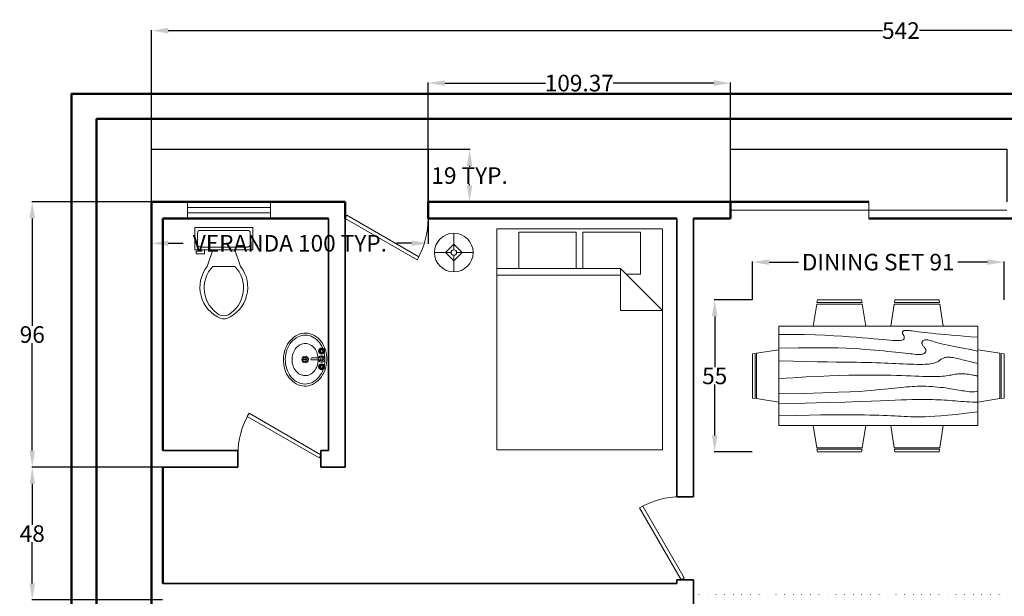
# Model space of a CAD drawing. Units: inches. Extents: x 910 to 1553, y 598 to 1516.
# Tile 5 of 6: x 912 to 1268, y 1307 to 1516. Entities that reach past the tile are written whole.
import ezdxf

# ---------------------------------------------------------------- set-up
doc = ezdxf.new("R2010")
doc.units = ezdxf.units.IN
doc.header["$MEASUREMENT"] = 0
doc.linetypes.add('ACAD_ISO07W100', pattern=[3, 0, -3])
for name, color, linetype, lineweight in [('A-ANNO-DIMS', 2, 'Continuous', 18), ('A-FLOR-BALC', 8, 'Continuous', 25), ('A-FLOR-OVHD', 8, 'ACAD_ISO07W100', 13), ('doors', 2, 'Continuous', 18), ('furniture', 11, 'Continuous', 18), ('Inner wall', 230, 'Continuous', 35), ('outer wall', 231, 'Continuous', 50), ('sanitory', 141, 'Continuous', 18), ('windows', 6, 'Continuous', 18)]:
    doc.layers.add(name, color=color, linetype=linetype, lineweight=lineweight)
doc.styles.get("Standard").update_dxf_attribs({"font": 'arial.ttf'})
doc.dimstyles.get("Standard").update_dxf_attribs({"dimtxt": 6, "dimasz": 6, "dimexe": 0.18, "dimexo": 0.0625, "dimgap": 0.09, "dimtad": 0, "dimtih": 1, "dimtoh": 1, "dimdec": 0, "dimzin": 0, "dimdsep": 46, "dimlunit": 3, "dimtxsty": 'Standard', "dimcen": 0.09, "dimadec": 0, "dimazin": 0, "dimtfac": 1, "dimtdec": 0, "dimtofl": 0, "dimtmove": 0, "dimatfit": 3, "dimfxl": 1, "dimtolj": 1, "dimtzin": 0, "dimarcsym": 0})

# ---------------------------------------------------------------- blocks, each defined once
blk = doc.blocks.new('*U5')
for p, q in [((0, 0), (0, -6)), ((-40, 0), (-40, -6))]:
    blk.add_line(p, q)
blk.add_lwpolyline([(0, 0), (-34.64, 20), (-35.52, 18.48), (-0.88, -1.52)], close=True)
blk.add_arc((0, 0), 40, 150, 180)
blk = doc.blocks.new('*U3')
for p, q in [((0, 0), (0, -6)), ((40, 0), (40, -6))]:
    blk.add_line(p, q)
blk.add_lwpolyline([(0, 0), (34.64, 20), (35.52, 18.48), (0.88, -1.52)], close=True)
blk.add_arc((0, 0), 40, 0, 30)
blk = doc.blocks.new('*U4')
for p, q in [((0, 0), (0, 6)), ((40, 0), (40, 6))]:
    blk.add_line(p, q)
blk.add_lwpolyline([(0, 0), (34.64, -20), (35.52, -18.48), (0.87, 1.52)], close=True)
blk.add_arc((0, 0), 40, 330, 0)
blk = doc.blocks.new('Faucet - Bathroom top')
for p, q in [((-4.107, 0.125), (-4.375, 0.125)), ((-3.75, 0.4788), (-3.75, 0.75)), ((-3.5, 0.482), (-3.5, 0.75)), ((-3.1461, 0.125), (-2.875, 0.125)), ((3.143, 0.125), (2.875, 0.125)), ((3.5, 0.4788), (3.5, 0.75)), ((3.75, 0.482), (3.75, 0.75)), ((4.1039, 0.125), (4.375, 0.125)), ((-4.1039, -0.125), (-4.375, -0.125)), ((-3.75, -0.4821), (-3.75, -0.75)), ((-3.5, -0.4789), (-3.5, -0.75)), ((-3.143, -0.125), (-2.875, -0.125)), ((-0.5, -0.8639), (-0.5, -4.5)), ((0.5, -4.5), (0.5, -0.8631)), ((3.1461, -0.125), (2.875, -0.125)), ((3.5, -0.4821), (3.5, -0.75)), ((3.75, -0.4789), (3.75, -0.75)), ((4.107, -0.125), (4.375, -0.125))]:
    blk.add_line(p, q)
for centre, radius in [((-3.625, 0), 1.375), ((-4.625, 0), 0.2795), ((-3.625, 0), 0.5), ((-3.625, 1), 0.2795), ((-2.625, 0), 0.2795), ((0, 0), 0.5), ((3.625, 0), 1.375), ((2.625, 0), 0.2795), ((3.625, 0), 0.5), ((3.625, 1), 0.2795), ((4.625, 0), 0.2795), ((-3.625, -1), 0.2795), ((3.625, -1), 0.2795)]:
    blk.add_circle(centre, radius)
for centre, radius, start, end in [((-3.625, 0), 1, 105.2407, 164.2093), ((-3.625, 0), 1, 16.44125, 74.07887), ((0, 0), 1.5, 289.6514, 250.3603), ((0, 0), 1, 300.3431, 239.7554), ((3.625, 0), 1, 106.12, 164.0884), ((3.625, 0), 1, 16.23422, 73.90469), ((-3.625, 0), 1, 196.2342, 253.9047), ((-3.625, 0), 1, 286.12, 344.0884), ((0, -4.5), 0.5, 180, 0), ((3.625, 0), 1, 196.4413, 254.0789), ((3.625, 0), 1, 285.2407, 344.2093)]:
    blk.add_arc(centre, radius, start, end)
blk = doc.blocks.new('Bed - Queen')
for p, q in [((0, -80.00003), (0, 0)), ((0, 0), (59.99999, 0)), ((59.99999, 0), (59.99999, -80.00003)), ((7.99999, -1.2), (28.79998, -1.2)), ((7.99999, -14.4), (7.99999, -1.2)), ((28.79998, -1.2), (28.79998, -14.4)), ((31.19999, -1.2), (51.99999, -1.2)), ((31.19999, -14.4), (31.19999, -1.2)), ((51.99999, -1.2), (51.99999, -16.4)), ((0, -14.4), (44.8, -14.4)), ((44.8, -16.8), (0, -16.8)), ((59.99999, -29.6), (44.8, -14.4)), ((44.8, -14.4), (44.8, -29.6)), ((51.99999, -16.4), (46.79936, -16.4)), ((44.8, -29.6), (59.99999, -29.6)), ((59.99999, -80.00003), (0, -80.00003))]:
    blk.add_line(p, q)
blk = doc.blocks.new('Lamp - Table')
for p, q in [((0, 7), (0, 1)), ((-1, 0), (-7, 0)), ((0, 3), (-3, 0)), ((-3, 0), (0, -3)), ((3, 0), (0, 3)), ((0, -3), (3, 0)), ((1, 0), (7, 0)), ((0, -1), (0, -7))]:
    blk.add_line(p, q)
for radius in [7, 1]:
    blk.add_circle((0, 0), radius)
blk = doc.blocks.new('Toilet - top')
for p, q in [((9.5, -6), (9.5, -2)), ((-10, -8.5), (-8, -8.5)), ((-10, -9.5), (-10, -8.5)), ((-7, -9.5), (-10, -9.5)), ((-8, -8.5), (-8, -8)), ((-7, -8), (-7, -9.5)), ((-4, -8), (-6, -14)), ((4, -8), (6, -14)), ((4, -14), (-4, -14))]:
    blk.add_line(p, q)
blk.add_lwpolyline([(10.5, -8), (10.5, 0), (-10.5, 0), (-10.5, -8)], close=True)
for points in [[(-9.5, -2), (-9.5, -6)], [(8.5, -1), (-8.5, -1)], [(-8.5, -7), (8.5, -7)]]:
    blk.add_lwpolyline(points)
for centre, radius, start, end in [((-8.62, -1.88), 0.884, 81.8699, 188.1301), ((8.62, -1.88), 0.884, 351.8699, 98.1301), ((-8.62, -6.12), 0.884, 171.8699, 278.1301), ((8.62, -6.12), 0.884, 261.8699, 8.1301), ((3.52, -21.58), 12.17, 141.4691, 247.9714), ((4.2, -21.82), 11.33, 136.3677, 238.9468), ((-3.52, -21.58), 12.17, 292.0284, 38.5307), ((-4.2, -21.82), 11.33, 301.053, 43.6321), ((0, -27.88), 4, 245.7318, 294.2682), ((0, -29), 4, 254.8605, 285.1395)]:
    blk.add_arc(centre, radius, start, end)
blk = doc.blocks.new('Dining Set - 36 x 72 in.')
for p, q in [((-22.2343, 26.00059), (-23.4847, 17.99762)), ((-22.2304, 26), (-5.7608, 26)), ((-22, 27.5), (-22.1562, 26.50042)), ((-5.8416, 26.5), (-22.1534, 26.5)), ((-22, 27.5), (-6, 27.5)), ((-5.8437, 26.49966), (-6, 27.5)), ((-4.5152, 17.99762), (-5.7655, 25.99926)), ((5.7657, 26.00059), (4.5153, 17.99762)), ((5.7696, 26), (22.2392, 26)), ((6, 27.5), (5.8438, 26.50042)), ((22.1584, 26.5), (5.8466, 26.5)), ((6, 27.5), (22, 27.5)), ((22.1563, 26.49966), (22, 27.5)), ((23.4848, 17.99762), (22.2345, 25.99926)), ((36, 18), (-36, 18)), ((-36, 18), (-36, -18)), ((36, -18), (36, 18)), ((-45.5, 8), (-44.5004, 8.15617)), ((-45.5, 8), (-45.5, -8)), ((-44.5, -8.15843), (-44.5, 8.15338)), ((-44.0006, 8.23428), (-35.9976, 9.48474)), ((-44, 8.23041), (-44, -8.23915)), ((44.0006, 8.23428), (35.9976, 9.48474)), ((44, 8.23041), (44, -8.23915)), ((44.5, -8.15843), (44.5, 8.15338)), ((45.5, 8), (44.5005, 8.15617)), ((45.5, 8), (45.5, -8)), ((-44.4997, -8.15631), (-45.5, -8)), ((-35.9976, -9.48476), (-43.9993, -8.2345)), ((35.9976, -9.48476), (43.9993, -8.2345)), ((44.4997, -8.15631), (45.5, -8)), ((-36, -18), (36, -18)), ((-22.2343, -26.0006), (-23.4847, -17.99762)), ((-4.5152, -17.99762), (-5.7655, -25.99928)), ((5.7657, -26.0006), (4.5153, -17.99762)), ((23.4848, -17.99762), (22.2345, -25.99928)), ((-22.2304, -26), (-5.7608, -26)), ((-22, -27.5), (-22.1562, -26.50044)), ((-5.8416, -26.5), (-22.1534, -26.5)), ((-22, -27.5), (-6, -27.5)), ((-5.8437, -26.49967), (-6, -27.5)), ((5.7696, -26), (22.2392, -26)), ((6, -27.5), (5.8438, -26.50044)), ((22.1584, -26.5), (5.8466, -26.5)), ((6, -27.5), (22, -27.5)), ((22.1563, -26.49967), (22, -27.5))]:
    blk.add_line(p, q)
for points in [[(-36, 15), (-31.1772, 14.97754), (-26.8079, 14.91406), (-22.8538, 14.81543), (-19.276, 14.6875), (-16.0362, 14.53613), (-13.0957, 14.36718), (-10.4159, 14.18652), (-7.9583, 14), (-5.6904, 13.81315), (-3.6035, 13.63021), (-1.6954, 13.45508), (0.0365, 13.29166), (1.5945, 13.14388), (2.9811, 13.01562), (4.1988, 12.9108), (5.25, 12.83333), (6.1393, 12.78613), (6.8802, 12.76823), (7.4883, 12.77767), (7.9792, 12.8125), (8.3685, 12.87077), (8.6719, 12.95052), (8.9049, 13.0498), (9.0833, 13.16666), (9.2205, 13.29899), (9.3216, 13.44401), (9.3895, 13.59879), (9.4271, 13.76041), (9.4373, 13.92594), (9.4232, 14.09245), (9.3875, 14.257), (9.3333, 14.41666), (9.2638, 14.56917), (9.1836, 14.71484), (9.0975, 14.85465), (9.0104, 14.98958), (8.9272, 15.1206), (8.8529, 15.2487), (8.7922, 15.37483), (8.75, 15.5), (8.7305, 15.62467), (8.7344, 15.74739), (8.7617, 15.86621), (8.8125, 15.97916), (8.8867, 16.08431), (8.9844, 16.17968), (9.1055, 16.26334), (9.25, 16.33333), (9.4189, 16.38802), (9.6172, 16.42708), (9.8506, 16.45052), (10.125, 16.45833), (10.4463, 16.45052), (10.8203, 16.42708), (11.2529, 16.38802), (11.75, 16.33333), (12.3184, 16.26318), (12.9694, 16.17838), (13.7151, 16.07991), (14.5677, 15.96875), (15.5395, 15.84586), (16.6426, 15.71224), (17.8893, 15.56884), (19.2917, 15.41666), (20.859, 15.25667), (22.5879, 15.08984), (24.4721, 14.91715), (26.5052, 14.73958), (28.6809, 14.5581), (30.9929, 14.3737), (33.4347, 14.18733), (36, 14)], [(-36, 10), (-28.9766, 10.14274), (-23.1725, 10.20442), (-18.4241, 10.19775), (-14.5677, 10.13541), (-11.4399, 10.03011), (-8.877, 9.89453), (-6.7154, 9.74137), (-4.7917, 9.58333), (-2.9698, 9.43082), (-1.2246, 9.28515), (0.4415, 9.14534), (2.026, 9.01041), (3.5266, 8.87939), (4.9408, 8.7513), (6.266, 8.62516), (7.5, 8.5), (8.6411, 8.37549), (9.6914, 8.2539), (10.6538, 8.13818), (11.5312, 8.03125), (12.3267, 7.93603), (13.043, 7.85547), (13.6831, 7.79248), (14.25, 7.75), (14.7471, 7.7303), (15.1797, 7.73307), (15.5537, 7.75732), (15.875, 7.80208), (16.1494, 7.86637), (16.3828, 7.94922), (16.5811, 8.04964), (16.75, 8.16666), (16.8944, 8.29915), (17.0143, 8.44531), (17.1089, 8.60319), (17.1771, 8.77083), (17.218, 8.94629), (17.2305, 9.1276), (17.2137, 9.31282), (17.1667, 9.5), (17.0895, 9.6875), (16.987, 9.875), (16.8649, 10.0625), (16.7292, 10.25), (16.5856, 10.4375), (16.4401, 10.625), (16.2985, 10.8125), (16.1667, 11), (16.05, 11.18733), (15.9518, 11.3737), (15.8752, 11.5581), (15.8229, 11.73958), (15.798, 11.91715), (15.8034, 12.08984), (15.842, 12.25667), (15.9167, 12.41666), (16.0295, 12.56836), (16.1784, 12.70833), (16.3605, 12.83268), (16.5729, 12.9375), (16.8127, 13.01888), (17.0768, 13.07291), (17.3625, 13.0957), (17.6667, 13.08333), (17.9894, 13.03312), (18.3418, 12.94726), (18.7382, 12.82918), (19.1927, 12.68229), (19.7195, 12.51001), (20.3327, 12.31575), (21.0465, 12.10294), (21.875, 11.875), (22.8357, 11.63354), (23.959, 11.37304), (25.2786, 11.08618), (26.8282, 10.76562), (28.6414, 10.40405), (30.752, 9.99414), (33.1936, 9.52856), (36, 9)], [(-36, 5.5), (-30.7157, 5.3348), (-26.069, 5.20963), (-21.9946, 5.11767), (-18.4271, 5.05208), (-15.3009, 5.00602), (-12.5508, 4.97265), (-10.1112, 4.94515), (-7.9167, 4.91666), (-5.909, 4.88167), (-4.0586, 4.83984), (-2.3429, 4.79215), (-0.7396, 4.73958), (0.7739, 4.6831), (2.22, 4.6237), (3.6213, 4.56233), (5, 4.5), (6.373, 4.43782), (7.7344, 4.3776), (9.0723, 4.32129), (10.375, 4.27083), (11.6309, 4.22819), (12.8281, 4.19531), (13.9551, 4.17415), (15, 4.16666), (15.954, 4.17448), (16.819, 4.19791), (17.6001, 4.23698), (18.3021, 4.29166), (18.9299, 4.36198), (19.4883, 4.44791), (19.9823, 4.54948), (20.4167, 4.66666), (20.7969, 4.79899), (21.1302, 4.94401), (21.4245, 5.09879), (21.6875, 5.26041), (21.9271, 5.42594), (22.1511, 5.59245), (22.3672, 5.757), (22.5834, 5.91666), (22.8065, 6.06868), (23.0404, 6.21093), (23.2879, 6.34147), (23.5521, 6.45833), (23.8358, 6.55957), (24.142, 6.64323), (24.4735, 6.70735), (24.8334, 6.75), (25.2235, 6.76969), (25.642, 6.76692), (26.0858, 6.74267), (26.5521, 6.69791), (27.0379, 6.63362), (27.5404, 6.55078), (28.0565, 6.45036), (28.5834, 6.33333), (29.1242, 6.19987), (29.7071, 6.04687), (30.3661, 5.87044), (31.1354, 5.66666), (32.0493, 5.43164), (33.142, 5.16146), (34.4475, 4.85221), (36, 4.5)], [(-36, -1), (-30.7915, -0.6591), (-26.0195, -0.38216), (-21.6519, -0.16284), (-17.6563, 0.00521), (-14.0005, 0.12833), (-10.6523, 0.21289), (-7.5796, 0.26522), (-4.75, 0.29166), (-2.134, 0.29793), (0.2878, 0.28711), (2.5317, 0.26163), (4.6146, 0.22396), (6.5529, 0.17651), (8.3633, 0.12174), (10.0623, 0.06209), (11.6667, 0), (13.1899, -0.06201), (14.6341, -0.1211), (15.9982, -0.17432), (17.2813, -0.21875), (18.4823, -0.25147), (19.6003, -0.26953), (20.6343, -0.27002), (21.5834, -0.25), (22.4481, -0.20768), (23.2357, -0.14584), (23.9549, -0.06836), (24.6146, 0.02083), (25.2235, 0.11784), (25.7904, 0.21875), (26.3241, 0.31966), (26.8334, 0.41666), (27.3265, 0.50618), (27.8099, 0.58593), (28.2894, 0.65397), (28.7709, 0.70833), (29.2601, 0.74707), (29.763, 0.76823), (30.2855, 0.76985), (30.8334, 0.75), (31.4088, 0.70784), (31.9994, 0.64713), (32.589, 0.57275), (33.1615, 0.48958), (33.7008, 0.4025), (34.1908, 0.3164), (34.6153, 0.23616), (34.9584, 0.16666), (35.2099, 0.11165), (35.3848, 0.07031), (35.504, 0.04069), (35.5886, 0.02083), (35.6594, 0.00879), (35.7377, 0.0026), (35.8442, 0.00032), (36, 0)], [(-36, -6.5), (-27.1843, -6.31267), (-20.084, -6.1263), (-14.469, -5.9419), (-10.1094, -5.76042), (-6.7752, -5.58285), (-4.2363, -5.41016), (-2.2629, -5.24333), (-0.625, -5.08334), (0.8708, -4.93099), (2.2715, -4.78646), (3.5872, -4.64974), (4.8281, -4.52084), (6.0046, -4.39974), (7.127, -4.28646), (8.2053, -4.18099), (9.25, -4.08334), (10.2705, -3.99382), (11.2734, -3.91407), (12.2647, -3.84603), (13.25, -3.79167), (14.2354, -3.75293), (15.2266, -3.73177), (16.2295, -3.73015), (17.25, -3.75), (18.2912, -3.79248), (19.3451, -3.85547), (20.4009, -3.93604), (21.4479, -4.03125), (22.4754, -4.13819), (23.4727, -4.25391), (24.4289, -4.37549), (25.3334, -4.5), (26.1785, -4.62492), (26.9694, -4.74935), (27.7145, -4.87281), (28.4219, -4.99479), (29.1, -5.11483), (29.7572, -5.23242), (30.4016, -5.34709), (31.0417, -5.45834), (31.6837, -5.56437), (32.3262, -5.65821), (32.9658, -5.73153), (33.599, -5.77604), (34.2224, -5.78345), (34.8327, -5.74545), (35.4264, -5.65373), (36, -5.5)], [(-36, -10), (-26.4022, -9.81299), (-18.4675, -9.62891), (-11.9839, -9.45069), (-6.7396, -9.28125), (-2.5226, -9.12354), (0.8789, -8.98047), (3.6769, -8.85498), (6.0833, -8.75), (8.2767, -8.66765), (10.3021, -8.60677), (12.1712, -8.56543), (13.8958, -8.54167), (15.4876, -8.53353), (16.9583, -8.53907), (18.3197, -8.55632), (19.5834, -8.58334), (20.7616, -8.61841), (21.8685, -8.66081), (22.9188, -8.71004), (23.9271, -8.76563), (24.9081, -8.82707), (25.8763, -8.89388), (26.8465, -8.96558), (27.8334, -9.04167), (28.8474, -9.12118), (29.8828, -9.20117), (30.93, -9.27824), (31.9792, -9.34896), (33.0205, -9.40991), (34.0443, -9.45768), (35.0407, -9.48885), (36, -9.5)], [(-36, -14.5), (-30.0881, -14.33513), (-25.0332, -14.21224), (-20.7312, -14.12647), (-17.0781, -14.07292), (-13.97, -14.04671), (-11.3027, -14.04297), (-8.9724, -14.05681), (-6.875, -14.08334), (-4.9224, -14.11833), (-3.0905, -14.16016), (-1.3709, -14.20785), (0.2448, -14.26042), (1.7647, -14.3169), (3.1973, -14.3763), (4.5507, -14.43767), (5.8333, -14.5), (7.0554, -14.5621), (8.235, -14.62175), (9.3922, -14.67652), (10.5469, -14.72396), (11.7192, -14.76164), (12.929, -14.78711), (14.1965, -14.79794), (15.5417, -14.79167), (16.9933, -14.76424), (18.6152, -14.70508), (20.4804, -14.60197), (22.6615, -14.44271), (25.2312, -14.21509), (28.2624, -13.9069), (31.8277, -13.50594), (36, -13)]]:
    blk.add_lwpolyline(points)
blk = doc.blocks.new('Sink - Oval top')
for p, q in [((-1, 0), (1, 0)), ((0, 1), (0, -1))]:
    blk.add_line(p, q)
for points in [[(-12.23, 0.39, 0.117634), (-11.46, -3.36, 0.104469), (-8.88, -6.8, 0.090016), (-5.08, -9.07, 0.08192), (-0.32, -10.02, 0.08192), (4.49, -9.38, 0.090016), (8.42, -7.36, 0.104469), (11.22, -4.09, 0.117634), (12.23, -0.39, 0.117634), (11.46, 3.36, 0.104469), (8.88, 6.8, 0.090016), (5.08, 9.07, 0.08192), (0.32, 10.02, 0.08192), (-4.49, 9.38, 0.090016), (-8.42, 7.36, 0.104469), (-11.22, 4.09, 0.117634)], [(-11.29, 0.16, 0.118622), (-10.52, -3.25, 0.104678), (-8.07, -6.36, 0.089562), (-4.54, -8.37, 0.081185), (-0.13, -9.15, 0.081185), (4.3, -8.49, 0.089562), (7.89, -6.58, 0.104678), (10.42, -3.55, 0.118622), (11.29, -0.16, 0.118622), (10.52, 3.25, 0.104678), (8.07, 6.36, 0.089562), (4.54, 8.37, 0.081185), (0.13, 9.15, 0.081185), (-4.3, 8.49, 0.089562), (-7.89, 6.58, 0.104678), (-10.42, 3.55, 0.118622)], [(-7.42, 0.08, 0.118283), (-6.91, -2.17, 0.104607), (-5.29, -4.21, 0.089718), (-2.97, -5.53, 0.081436), (-0.07, -6.04, 0.081436), (2.84, -5.59, 0.089718), (5.2, -4.33, 0.104607), (6.86, -2.32, 0.118283), (7.42, -0.08, 0.118283), (6.91, 2.17, 0.104607), (5.29, 4.21, 0.089718), (2.97, 5.53, 0.081436), (0.07, 6.04, 0.081436), (-2.84, 5.59, 0.089718), (-5.2, 4.33, 0.104607), (-6.86, 2.32, 0.118283)]]:
    blk.add_lwpolyline(points, format="xyb", close=True)
for radius in [1.5, 1]:
    blk.add_circle((0, 0), radius)
blk = doc.blocks.new('WIN-30X6')
for p, q in [((0, 6), (30, 6)), ((0, 0), (0, 6)), ((0, 4), (30, 4)), ((30, 6), (30, 0)), ((30, 2), (0, 2)), ((30, 0), (0, 0))]:
    blk.add_line(p, q)
blk = doc.blocks.new('VERANDA-EDGE-SHALLOW')
for p, q in [((0, 0), (0, 18.99)), ((0, 18.99), (100, 18.99)), ((100, 18.99), (100, 0))]:
    blk.add_line(p, q)
blk = doc.blocks.new('*D45')
at = {"layer": 'A-ANNO-DIMS', "color": 0, "lineweight": -2, "transparency": 16777216}
for p, q in [((959.7, 1449.91), (959.7, 1434.79)), ((1059.7, 1449.91), (1059.7, 1434.79)), ((965.7, 1434.97), (971.1, 1434.97)), ((1053.7, 1434.97), (1048.31, 1434.97))]:
    blk.add_line(p, q, dxfattribs=at)
for points in [[(965.7, 1435.97), (965.7, 1433.97), (959.7, 1434.97)], [(1053.7, 1435.97), (1053.7, 1433.97), (1059.7, 1434.97)]]:
    blk.add_solid(points, dxfattribs=at)
at = {"layer": 'Defpoints', "color": 0, "lineweight": -2, "transparency": 16777216}
for p in [(959.7, 1449.97), (1059.7, 1449.97), (1059.7, 1434.97)]:
    blk.add_point(p, dxfattribs=at)
at = {"layer": 'A-ANNO-DIMS', "color": 0, "transparency": 16777216, "insert": (1009.7, 1434.97), "char_height": 6, "attachment_point": 5}
blk.add_mtext('\\A1;VERANDA 100 TYP.', dxfattribs=at)
blk = doc.blocks.new('*D46')
at = {"layer": 'A-ANNO-DIMS', "color": 0, "lineweight": -2, "transparency": 16777216}
for p, q in [((1059.76, 1468.95), (1074.88, 1468.95)), ((1074.7, 1462.95), (1074.7, 1462.62)), ((1074.7, 1455.97), (1074.7, 1456.31)), ((1059.76, 1449.97), (1074.88, 1449.97))]:
    blk.add_line(p, q, dxfattribs=at)
for points in [[(1073.7, 1462.95), (1075.7, 1462.95), (1074.7, 1468.95)], [(1073.7, 1455.97), (1075.7, 1455.97), (1074.7, 1449.97)]]:
    blk.add_solid(points, dxfattribs=at)
at = {"layer": 'Defpoints', "color": 0, "lineweight": -2, "transparency": 16777216}
for p in [(1059.7, 1468.95), (1074.7, 1468.95), (1059.7, 1449.97)]:
    blk.add_point(p, dxfattribs=at)
at = {"layer": 'A-ANNO-DIMS', "color": 0, "transparency": 16777216, "insert": (1074.7, 1459.46), "char_height": 6, "attachment_point": 5}
blk.add_mtext('\\A1;19 TYP.', dxfattribs=at)
blk = doc.blocks.new('*D53')
at = {"layer": 'A-ANNO-DIMS', "color": 0, "lineweight": -2, "transparency": 16777216}
for p, q in [((1177, 1414.56), (1177, 1428.33)), ((1183, 1428.15), (1193.69, 1428.15)), ((1262, 1428.15), (1251.31, 1428.15)), ((1268, 1414.56), (1268, 1428.33))]:
    blk.add_line(p, q, dxfattribs=at)
for points in [[(1183, 1429.15), (1183, 1427.15), (1177, 1428.15)], [(1262, 1429.15), (1262, 1427.15), (1268, 1428.15)]]:
    blk.add_solid(points, dxfattribs=at)
at = {"layer": 'Defpoints', "color": 0, "lineweight": -2, "transparency": 16777216}
for p in [(1268, 1428.15), (1177, 1414.5), (1268, 1414.5)]:
    blk.add_point(p, dxfattribs=at)
at = {"layer": 'A-ANNO-DIMS', "color": 0, "transparency": 16777216, "insert": (1222.5, 1428.15), "char_height": 6, "attachment_point": 5}
blk.add_mtext('\\A1;DINING SET 91', dxfattribs=at)
blk = doc.blocks.new('*D54')
at = {"layer": 'A-ANNO-DIMS', "color": 0, "lineweight": -2, "transparency": 16777216}
for p, q in [((1176.94, 1414.5), (1163.17, 1414.5)), ((1163.35, 1408.5), (1163.35, 1390.14)), ((1163.35, 1365.5), (1163.35, 1383.86)), ((1176.94, 1359.5), (1163.17, 1359.5))]:
    blk.add_line(p, q, dxfattribs=at)
for points in [[(1162.35, 1408.5), (1164.35, 1408.5), (1163.35, 1414.5)], [(1162.35, 1365.5), (1164.35, 1365.5), (1163.35, 1359.5)]]:
    blk.add_solid(points, dxfattribs=at)
at = {"layer": 'Defpoints', "color": 0, "lineweight": -2, "transparency": 16777216}
for p in [(1163.35, 1414.5), (1177, 1414.5), (1177, 1359.5)]:
    blk.add_point(p, dxfattribs=at)
at = {"layer": 'A-ANNO-DIMS', "color": 0, "transparency": 16777216, "insert": (1163.35, 1387), "char_height": 6, "attachment_point": 5}
blk.add_mtext('\\A1;55', dxfattribs=at)
blk = doc.blocks.new('*D55')
at = {"layer": 'A-ANNO-DIMS', "color": 0, "lineweight": -2, "transparency": 16777216}
for p, q in [((959.7, 1469.02), (959.7, 1512.08)), ((965.7, 1511.9), (1224.01, 1511.9)), ((1495.7, 1511.9), (1237.39, 1511.9)), ((1501.7, 1469.02), (1501.7, 1512.08))]:
    blk.add_line(p, q, dxfattribs=at)
for points in [[(965.7, 1512.9), (965.7, 1510.9), (959.7, 1511.9)], [(1495.7, 1512.9), (1495.7, 1510.9), (1501.7, 1511.9)]]:
    blk.add_solid(points, dxfattribs=at)
at = {"layer": 'Defpoints', "color": 0, "lineweight": -2, "transparency": 16777216}
for p in [(1501.7, 1511.9), (959.7, 1468.95), (1501.7, 1468.95)]:
    blk.add_point(p, dxfattribs=at)
at = {"layer": 'A-ANNO-DIMS', "color": 0, "transparency": 16777216, "insert": (1230.7, 1511.9), "char_height": 6, "attachment_point": 5}
blk.add_mtext('\\A1;542', dxfattribs=at)
blk = doc.blocks.new('*D69')
at = {"layer": 'A-ANNO-DIMS', "color": 0, "lineweight": -2, "transparency": 16777216}
for p, q in [((963.64, 1353.97), (916.34, 1353.97)), ((916.52, 1347.97), (916.52, 1333.12)), ((916.52, 1311.97), (916.52, 1326.82)), ((963.64, 1305.97), (916.34, 1305.97))]:
    blk.add_line(p, q, dxfattribs=at)
for points in [[(915.52, 1347.97), (917.52, 1347.97), (916.52, 1353.97)], [(915.52, 1311.97), (917.52, 1311.97), (916.52, 1305.97)]]:
    blk.add_solid(points, dxfattribs=at)
at = {"layer": 'Defpoints', "color": 0, "lineweight": -2, "transparency": 16777216}
for p in [(916.52, 1353.97), (963.7, 1353.97), (963.7, 1305.97)]:
    blk.add_point(p, dxfattribs=at)
at = {"layer": 'A-ANNO-DIMS', "color": 0, "transparency": 16777216, "insert": (916.52, 1329.97), "char_height": 6, "attachment_point": 5}
blk.add_mtext('\\A1;48', dxfattribs=at)
blk = doc.blocks.new('*D70')
at = {"layer": 'A-ANNO-DIMS', "color": 0, "lineweight": -2, "transparency": 16777216}
for p, q in [((959.64, 1449.97), (916.34, 1449.97)), ((916.52, 1443.97), (916.52, 1405.12)), ((916.52, 1359.97), (916.52, 1398.82)), ((963.64, 1353.97), (916.34, 1353.97))]:
    blk.add_line(p, q, dxfattribs=at)
for points in [[(915.52, 1443.97), (917.52, 1443.97), (916.52, 1449.97)], [(915.52, 1359.97), (917.52, 1359.97), (916.52, 1353.97)]]:
    blk.add_solid(points, dxfattribs=at)
at = {"layer": 'Defpoints', "color": 0, "lineweight": -2, "transparency": 16777216}
for p in [(916.52, 1449.97), (959.7, 1449.97), (963.7, 1353.97)]:
    blk.add_point(p, dxfattribs=at)
at = {"layer": 'A-ANNO-DIMS', "color": 0, "transparency": 16777216, "insert": (916.52, 1401.97), "char_height": 6, "attachment_point": 5}
blk.add_mtext('\\A1;96', dxfattribs=at)
blk = doc.blocks.new('*D86')
at = {"layer": 'A-ANNO-DIMS', "color": 0, "lineweight": -2, "transparency": 16777216}
for p, q in [((1059.7, 1450.03), (1059.7, 1493.1)), ((1065.7, 1492.92), (1102.12, 1492.92)), ((1163.07, 1492.92), (1126.65, 1492.92)), ((1169.07, 1450.03), (1169.07, 1493.1))]:
    blk.add_line(p, q, dxfattribs=at)
for points in [[(1065.7, 1493.92), (1065.7, 1491.92), (1059.7, 1492.92)], [(1163.07, 1493.92), (1163.07, 1491.92), (1169.07, 1492.92)]]:
    blk.add_solid(points, dxfattribs=at)
at = {"layer": 'Defpoints', "color": 0, "lineweight": -2, "transparency": 16777216}
for p in [(1169.07, 1492.92), (1059.7, 1449.97), (1169.07, 1449.97)]:
    blk.add_point(p, dxfattribs=at)
at = {"layer": 'A-ANNO-DIMS', "color": 0, "transparency": 16777216, "insert": (1114.38, 1492.92), "char_height": 6, "attachment_point": 5}
blk.add_mtext('\\A1;109.37', dxfattribs=at)

msp = doc.modelspace()

# ---------------------------------------------------------------- linework, layer by layer
at = {"layer": 'A-FLOR-OVHD'}
msp.add_line((1281.7, 1307.89), (1155.7, 1307.89), dxfattribs=at)
at = {"layer": 'doors'}
for p, q in [((1169.066, 1449.969), (1219.066, 1449.969)), ((1219.066, 1449.969), (1219.066, 1443.969)), ((1169.078, 1446.969), (1219.066, 1446.969)), ((1219.066, 1446.969), (1269.066, 1446.969)), ((1269.066, 1443.969), (1219.066, 1443.969))]:
    msp.add_line(p, q, dxfattribs=at)
at = {"layer": 'Inner wall'}
for p, q in [((1023.7, 1443.969), (1023.7, 1359.969)), ((1029.7, 1443.969), (1029.7, 1353.969)), ((1149.7, 1443.969), (1149.7, 1343.296)), ((1155.7, 1443.969), (1155.7, 1343.296)), ((1155.7, 1443.969), (1155.7, 1343.296)), ((990.908, 1359.969), (963.7, 1359.969)), ((1023.7, 1359.969), (1020.908, 1359.969)), ((990.908, 1353.969), (963.7, 1353.969)), ((1029.7, 1353.969), (1020.908, 1353.969)), ((1149.7, 1311.969), (963.7, 1311.969)), ((1149.7, 1313.296), (1149.7, 1311.969)), ((1155.7, 1313.296), (1155.7, 1311.969)), ((1155.7, 1313.296), (1155.7, 1218.289)), ((1155.7, 1313.296), (1155.7, 1218.289))]:
    msp.add_line(p, q, dxfattribs=at)
for points in [[(990.908, 1353.969), (990.908, 1359.969)], [(1020.908, 1359.969), (1020.908, 1353.969)], [(1149.7, 1343.296), (1155.7, 1343.296)], [(1155.7, 1313.296), (1149.7, 1313.296)]]:
    msp.add_lwpolyline(points, dxfattribs=at)
at = {"layer": 'outer wall'}
for p, q in [((1521.7, 1479.969), (939.7, 1479.969)), ((939.7, 1479.969), (939.7, 633.969)), ((959.7, 1449.969), (959.7, 681.969)), ((963.7, 1449.969), (959.7, 1449.969)), ((1029.7, 1449.969), (963.7, 1449.969)), ((1029.7, 1449.969), (963.7, 1449.969)), ((1219.066, 1449.969), (1059.7, 1449.969)), ((1219.066, 1449.969), (1059.7, 1449.969)), ((1059.7, 1449.969), (1169.066, 1449.969)), ((1169.089, 1443.969), (1169.066, 1449.969)), ((963.7, 1443.969), (963.7, 1359.969)), ((1023.7, 1443.969), (963.7, 1443.969)), ((1149.7, 1443.969), (1059.7, 1443.969)), ((1169.089, 1443.969), (1155.7, 1443.969)), ((1281.7, 1443.969), (1219.066, 1443.969)), ((963.7, 1353.969), (963.7, 1311.969))]:
    msp.add_line(p, q, dxfattribs=at)
msp.add_lwpolyline([(1530.7, 1488.969), (930.7, 1488.969), (930.7, 624.969), (1530.7, 624.969)], close=True, dxfattribs=at)
for points in [[(1029.7, 1443.969), (1029.7, 1449.969)], [(1059.7, 1449.969), (1059.7, 1443.969)]]:
    msp.add_lwpolyline(points, dxfattribs=at)

# ---------------------------------------------------------------- block references
at = {"layer": 'A-FLOR-BALC'}
for p in [(959.7, 1449.969), (1169.066, 1449.969)]:
    msp.add_blockref('VERANDA-EDGE-SHALLOW', p, dxfattribs=at)
at = {"layer": 'doors', "xscale": 0.75, "yscale": 0.75, "zscale": 0.75}
for name, p in [('*U4', (1029.7, 1443.969)), ('*U5', (1020.908, 1358.469))]:
    msp.add_blockref(name, p, dxfattribs=at)
at = {"layer": 'doors', "xscale": 0.75, "yscale": 0.75, "zscale": 0.75, "rotation": 90}
msp.add_blockref('*U3', (1151.2, 1313.296), dxfattribs=at)
at = {"layer": 'furniture'}
for name, p in [('Bed - Queen', (1084.502, 1440.214)), ('Lamp - Table', (1069, 1431.613)), ('Dining Set - 36 x 72 in.', (1222.5, 1387))]:
    msp.add_blockref(name, p, dxfattribs=at)
at = {"layer": 'sanitory'}
msp.add_blockref('Toilet - top', (985.818, 1440.622), dxfattribs=at)
at = {"layer": 'sanitory', "xscale": 0.7833329843755676, "yscale": 0.7833329843755676, "zscale": 0.7833329843755676}
for name, p, rotation in [('Sink - Oval top', (1015.208, 1392.902), 90), ('Faucet - Bathroom top', (1021.175, 1393.145), 270)]:
    msp.add_blockref(name, p, dxfattribs=dict(at, rotation=rotation))
at = {"layer": 'windows', "rotation": 180}
msp.add_blockref('WIN-30X6', (1002.662, 1449.969), dxfattribs=at)

# ---------------------------------------------------------------- dimensions: what is measured, and where the dimension line sits
at = {"layer": 'A-ANNO-DIMS'}
for base, p1, p2, override, picture, middle in [((1501.7, 1511.905), (959.7, 1468.955), (1501.7, 1468.955), {"dimdec": 0, "dimlfac": 1, "dimrnd": 0, "dimzin": 0, "dimdsep": 46, "dimlunit": 2}, '*D55', (1230.7, 1511.905)), ((1169.066, 1492.919), (1059.7, 1449.969), (1169.066, 1449.969), {"dimdec": 2, "dimlfac": 1, "dimrnd": 0, "dimzin": 0, "dimdsep": 46, "dimlunit": 2}, '*D86', (1114.383, 1492.919))]:
    dim = msp.add_linear_dim(base=base, p1=p1, p2=p2, dimstyle='Standard', override=override, dxfattribs=at)
    dim.commit()
    dim.dimension.update_dxf_attribs({"geometry": picture, "text_midpoint": middle})
dim = msp.add_linear_dim(base=(1074.7, 1468.955), p1=(1059.7, 1449.969), p2=(1059.7, 1468.955), angle=90, text='<> TYP.', dimstyle='Standard', override={"dimdec": 0, "dimlfac": 1, "dimrnd": 0, "dimzin": 0, "dimdsep": 46, "dimlunit": 2}, dxfattribs=at)
dim.commit()
dim.dimension.update_dxf_attribs({"geometry": '*D46', "text_midpoint": (1074.7, 1459.462)})
for base, p1, p2, picture, middle in [((916.52, 1449.969), (963.7, 1353.969), (959.7, 1449.969), '*D70', (916.52, 1401.969)), ((1163.35, 1414.5), (1177, 1359.5), (1177, 1414.5), '*D54', (1163.35, 1387)), ((916.52, 1353.969), (963.7, 1305.969), (963.7, 1353.969), '*D69', (916.52, 1329.969))]:
    dim = msp.add_linear_dim(base=base, p1=p1, p2=p2, angle=90, dimstyle='Standard', override={"dimdec": 0, "dimlfac": 1, "dimrnd": 0, "dimzin": 0, "dimdsep": 46, "dimlunit": 2}, dxfattribs=at)
    dim.commit()
    dim.dimension.update_dxf_attribs({"geometry": picture, "text_midpoint": middle})
for base, p1, p2, text, picture, middle in [((1059.7, 1434.969), (959.7, 1449.969), (1059.7, 1449.969), 'VERANDA <> TYP.', '*D45', (1009.7, 1434.969)), ((1268, 1428.15), (1177, 1414.5), (1268, 1414.5), 'DINING SET <>', '*D53', (1222.5, 1428.15))]:
    dim = msp.add_linear_dim(base=base, p1=p1, p2=p2, text=text, dimstyle='Standard', override={"dimdec": 0, "dimlfac": 1, "dimrnd": 0, "dimzin": 0, "dimdsep": 46, "dimlunit": 2}, dxfattribs=at)
    dim.commit()
    dim.dimension.update_dxf_attribs({"geometry": picture, "text_midpoint": middle})

doc.saveas('drawing.dxf')
